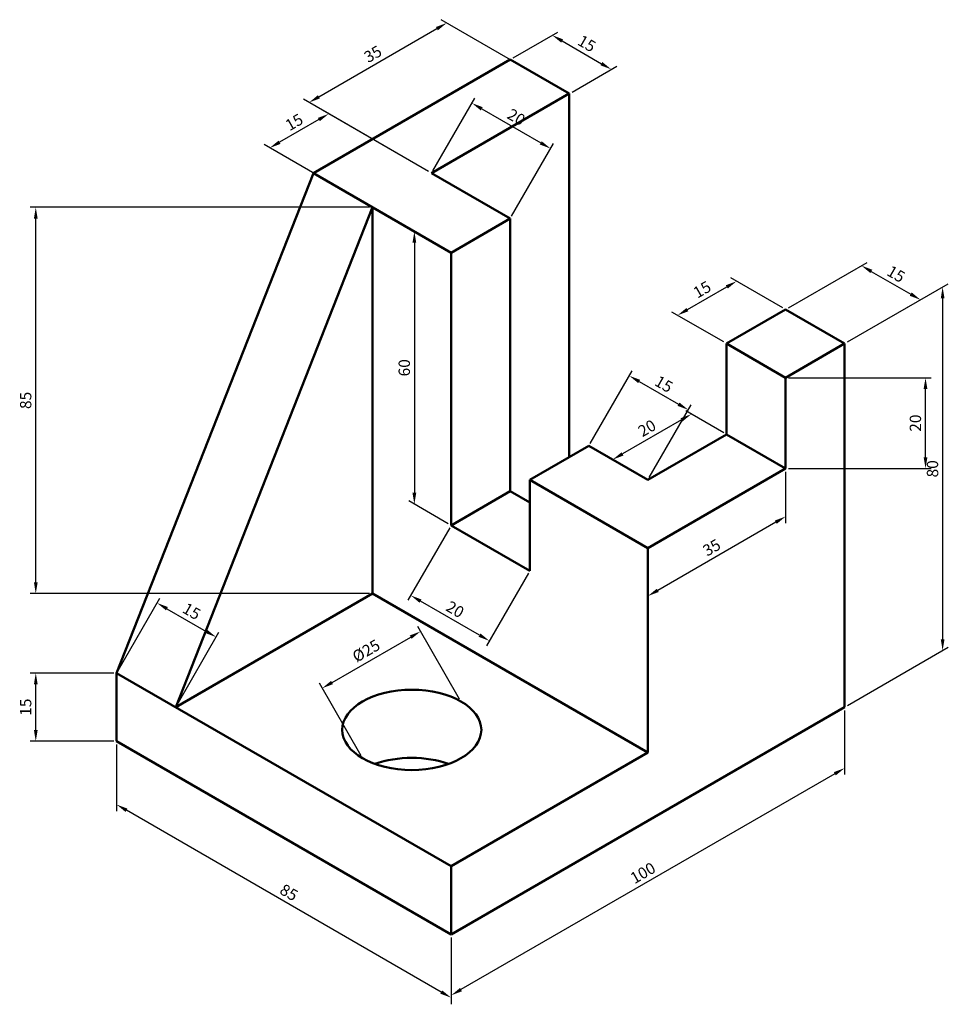
# Model space of a CAD drawing. Units: millimetres. Extents: x 1462 to 1666, y 2377 to 2594.
import ezdxf

# ---------------------------------------------------------------- set-up
doc = ezdxf.new("R2010")
doc.units = ezdxf.units.MM
doc.layers.add('M-DIMS', color=2, linetype='Continuous', lineweight=25)
doc.layers.add('M-OUTL', color=7, linetype='Continuous', lineweight=50)
doc.styles.get("Standard").update_dxf_attribs({"font": 'arial.ttf'})
doc.dimstyles.new('ISO-25', dxfattribs={"dimtxt": 2.5, "dimasz": 2.5, "dimexe": 1.25, "dimexo": 0.625, "dimtad": 1, "dimtxsty": 'Standard', "dimcen": 2.5, "dimadec": 0, "dimazin": 0, "dimtfac": 1, "dimtmove": 0, "dimatfit": 3, "dimfxl": 1, "dimarcsym": 0})

# ---------------------------------------------------------------- blocks, each defined once
blk = doc.blocks.new('*D1')
at = {"layer": 'Defpoints', "color": 0, "transparency": 16777216}
for p in [(1643.58, 2522.67), (1665.14, 2455.12), (1643.58, 2442.67)]:
    blk.add_point(p, dxfattribs=at)
at = {"layer": 'M-DIMS', "color": 0, "lineweight": -2, "transparency": 16777216}
for p, q in [((1644.2, 2523.03), (1666.39, 2535.85)), ((1665.14, 2532.62), (1665.14, 2457.62)), ((1644.2, 2443.03), (1666.39, 2455.85))]:
    blk.add_line(p, q, dxfattribs=at)
at = {"layer": 'M-DIMS', "color": 0, "transparency": 16777216}
for points in [[(1664.73, 2532.62), (1665.56, 2532.62), (1665.14, 2535.12)], [(1664.73, 2457.62), (1665.56, 2457.62), (1665.14, 2455.12)]]:
    blk.add_solid(points, dxfattribs=at)
at = {"layer": 'M-DIMS', "color": 0, "transparency": 16777216, "insert": (1663.24, 2495.12), "char_height": 2.5, "attachment_point": 5, "rotation": 90}
blk.add_mtext('80', dxfattribs=at)
blk = doc.blocks.new('*D2')
at = {"layer": 'Defpoints', "color": 0, "transparency": 16777216}
for p in [(1660.28, 2532.31), (1630.59, 2530.17), (1643.58, 2522.67)]:
    blk.add_point(p, dxfattribs=at)
at = {"layer": 'M-DIMS', "color": 0, "lineweight": -2, "transparency": 16777216}
for p, q in [((1631.21, 2530.53), (1648.54, 2540.54)), ((1649.45, 2538.56), (1658.11, 2533.56)), ((1644.2, 2523.03), (1661.53, 2533.04))]:
    blk.add_line(p, q, dxfattribs=at)
at = {"layer": 'M-DIMS', "color": 0, "transparency": 16777216}
for points in [[(1649.66, 2538.93), (1649.24, 2538.2), (1647.29, 2539.81)], [(1658.32, 2533.93), (1657.9, 2533.2), (1660.28, 2532.31)]]:
    blk.add_solid(points, dxfattribs=at)
at = {"layer": 'M-DIMS', "color": 0, "transparency": 16777216, "insert": (1654.73, 2537.71), "char_height": 2.5, "attachment_point": 5, "rotation": 330}
blk.add_mtext('15', dxfattribs=at)
blk = doc.blocks.new('*D3')
at = {"layer": 'Defpoints', "color": 0, "transparency": 16777216}
for p in [(1619.8, 2536.4), (1630.59, 2530.17), (1617.6, 2522.67)]:
    blk.add_point(p, dxfattribs=at)
at = {"layer": 'M-DIMS', "color": 0, "lineweight": -2, "transparency": 16777216}
for p, q in [((1608.98, 2530.15), (1617.64, 2535.15)), ((1629.96, 2530.53), (1618.55, 2537.12)), ((1616.97, 2523.03), (1605.56, 2529.62))]:
    blk.add_line(p, q, dxfattribs=at)
at = {"layer": 'M-DIMS', "color": 0, "transparency": 16777216}
for points in [[(1617.43, 2535.51), (1617.85, 2534.79), (1619.8, 2536.4)], [(1608.77, 2530.51), (1609.19, 2529.79), (1606.81, 2528.9)]]:
    blk.add_solid(points, dxfattribs=at)
at = {"layer": 'M-DIMS', "color": 0, "transparency": 16777216, "insert": (1612.36, 2534.3), "char_height": 2.5, "attachment_point": 5, "rotation": 30}
blk.add_mtext('15', dxfattribs=at)
blk = doc.blocks.new('*D4')
at = {"layer": 'Defpoints', "color": 0, "transparency": 16777216}
for p in [(1617.6, 2502.67), (1592.53, 2497.15), (1600.28, 2492.67)]:
    blk.add_point(p, dxfattribs=at)
at = {"layer": 'M-DIMS', "color": 0, "lineweight": -2, "transparency": 16777216}
for p, q in [((1616.97, 2503.03), (1608.6, 2507.87)), ((1607.68, 2505.9), (1594.69, 2498.4)), ((1599.65, 2493.03), (1591.28, 2497.87))]:
    blk.add_line(p, q, dxfattribs=at)
at = {"layer": 'M-DIMS', "color": 0, "transparency": 16777216}
for points in [[(1607.48, 2506.26), (1607.89, 2505.54), (1609.85, 2507.15)], [(1594.49, 2498.76), (1594.9, 2498.04), (1592.53, 2497.15)]]:
    blk.add_solid(points, dxfattribs=at)
at = {"layer": 'M-DIMS', "color": 0, "transparency": 16777216, "insert": (1600.24, 2503.79), "char_height": 2.5, "attachment_point": 5, "rotation": 30}
blk.add_mtext('20', dxfattribs=at)
blk = doc.blocks.new('*D5')
at = {"layer": 'Defpoints', "color": 0, "transparency": 16777216}
for p in [(1517.05, 2565.73), (1552.65, 2560.17), (1539.66, 2552.67)]:
    blk.add_point(p, dxfattribs=at)
at = {"layer": 'M-DIMS', "color": 0, "lineweight": -2, "transparency": 16777216}
for p, q in [((1527.87, 2571.98), (1519.21, 2566.98)), ((1552.02, 2560.53), (1528.79, 2573.95)), ((1539.03, 2553.03), (1515.8, 2566.45))]:
    blk.add_line(p, q, dxfattribs=at)
at = {"layer": 'M-DIMS', "color": 0, "transparency": 16777216}
for points in [[(1527.66, 2572.34), (1528.08, 2571.62), (1530.04, 2573.23)], [(1519, 2567.34), (1519.42, 2566.62), (1517.05, 2565.73)]]:
    blk.add_solid(points, dxfattribs=at)
at = {"layer": 'M-DIMS', "color": 0, "transparency": 16777216, "insert": (1522.59, 2571.12), "char_height": 2.5, "attachment_point": 5, "rotation": 30}
blk.add_mtext('15', dxfattribs=at)
blk = doc.blocks.new('*D6')
at = {"layer": 'Defpoints', "color": 0, "transparency": 16777216}
for p in [(1556.02, 2593.23), (1582.96, 2577.67), (1552.65, 2560.17)]:
    blk.add_point(p, dxfattribs=at)
at = {"layer": 'M-DIMS', "color": 0, "lineweight": -2, "transparency": 16777216}
for p, q in [((1582.33, 2578.03), (1554.77, 2593.95)), ((1527.87, 2576.98), (1553.85, 2591.98)), ((1552.02, 2560.53), (1524.46, 2576.45))]:
    blk.add_line(p, q, dxfattribs=at)
at = {"layer": 'M-DIMS', "color": 0, "transparency": 16777216}
for points in [[(1553.64, 2592.34), (1554.06, 2591.62), (1556.02, 2593.23)], [(1527.66, 2577.34), (1528.08, 2576.62), (1525.71, 2575.73)]]:
    blk.add_solid(points, dxfattribs=at)
at = {"layer": 'M-DIMS', "color": 0, "transparency": 16777216, "insert": (1539.91, 2586.12), "char_height": 2.5, "attachment_point": 5, "rotation": 30}
blk.add_mtext('35', dxfattribs=at)
blk = doc.blocks.new('*D7')
at = {"layer": 'Defpoints', "color": 0, "transparency": 16777216}
for p in [(1569.97, 2585.17), (1592.22, 2583.02), (1582.96, 2577.67)]:
    blk.add_point(p, dxfattribs=at)
at = {"layer": 'M-DIMS', "color": 0, "lineweight": -2, "transparency": 16777216}
for p, q in [((1570.59, 2585.53), (1580.48, 2591.24)), ((1581.39, 2589.27), (1590.05, 2584.27)), ((1583.58, 2578.03), (1593.47, 2583.74))]:
    blk.add_line(p, q, dxfattribs=at)
at = {"layer": 'M-DIMS', "color": 0, "transparency": 16777216}
for points in [[(1581.6, 2589.63), (1581.19, 2588.91), (1579.23, 2590.52)], [(1590.26, 2584.63), (1589.85, 2583.91), (1592.22, 2583.02)]]:
    blk.add_solid(points, dxfattribs=at)
at = {"layer": 'M-DIMS', "color": 0, "transparency": 16777216, "insert": (1586.68, 2588.42), "char_height": 2.5, "attachment_point": 5, "rotation": 330}
blk.add_mtext('15', dxfattribs=at)
blk = doc.blocks.new('*D8')
at = {"layer": 'Defpoints', "color": 0, "transparency": 16777216}
for p in [(1556.98, 2542.67), (1548.88, 2487.35), (1556.98, 2482.67)]:
    blk.add_point(p, dxfattribs=at)
at = {"layer": 'M-DIMS', "color": 0, "lineweight": -2, "transparency": 16777216}
for p, q in [((1556.35, 2543.03), (1547.63, 2548.07)), ((1548.88, 2544.85), (1548.88, 2489.85)), ((1556.35, 2483.03), (1547.63, 2488.07))]:
    blk.add_line(p, q, dxfattribs=at)
at = {"layer": 'M-DIMS', "color": 0, "transparency": 16777216}
for points in [[(1548.46, 2544.85), (1549.3, 2544.85), (1548.88, 2547.35)], [(1548.46, 2489.85), (1549.3, 2489.85), (1548.88, 2487.35)]]:
    blk.add_solid(points, dxfattribs=at)
at = {"layer": 'M-DIMS', "color": 0, "transparency": 16777216, "insert": (1546.98, 2517.35), "char_height": 2.5, "attachment_point": 5, "rotation": 90}
blk.add_mtext('60', dxfattribs=at)
blk = doc.blocks.new('*D9')
at = {"layer": 'Defpoints', "color": 0, "transparency": 16777216}
for p in [(1630.59, 2495.17), (1600.28, 2477.67), (1600.28, 2467.12)]:
    blk.add_point(p, dxfattribs=at)
at = {"layer": 'M-DIMS', "color": 0, "lineweight": -2, "transparency": 16777216}
for p, q in [((1630.59, 2494.45), (1630.59, 2483.17)), ((1628.42, 2483.37), (1602.44, 2468.37)), ((1600.28, 2476.95), (1600.28, 2465.67))]:
    blk.add_line(p, q, dxfattribs=at)
at = {"layer": 'M-DIMS', "color": 0, "transparency": 16777216}
for points in [[(1628.21, 2483.73), (1628.63, 2483.01), (1630.59, 2484.62)], [(1602.23, 2468.73), (1602.65, 2468.01), (1600.28, 2467.12)]]:
    blk.add_solid(points, dxfattribs=at)
at = {"layer": 'M-DIMS', "color": 0, "transparency": 16777216, "insert": (1614.48, 2477.52), "char_height": 2.5, "attachment_point": 5, "rotation": 30}
blk.add_mtext('35', dxfattribs=at)
blk = doc.blocks.new('*D10')
at = {"layer": 'Defpoints', "color": 0, "transparency": 16777216}
for p in [(1643.58, 2442.67), (1556.98, 2392.67), (1556.98, 2379.26)]:
    blk.add_point(p, dxfattribs=at)
at = {"layer": 'M-DIMS', "color": 0, "lineweight": -2, "transparency": 16777216}
for p, q in [((1643.58, 2441.95), (1643.58, 2427.82)), ((1641.41, 2428.01), (1559.14, 2380.51)), ((1556.98, 2391.95), (1556.98, 2377.82))]:
    blk.add_line(p, q, dxfattribs=at)
at = {"layer": 'M-DIMS', "color": 0, "transparency": 16777216}
for points in [[(1641.2, 2428.37), (1641.62, 2427.65), (1643.58, 2429.26)], [(1558.93, 2380.87), (1559.35, 2380.15), (1556.98, 2379.26)]]:
    blk.add_solid(points, dxfattribs=at)
at = {"layer": 'M-DIMS', "color": 0, "transparency": 16777216, "insert": (1599.33, 2405.91), "char_height": 2.5, "attachment_point": 5, "rotation": 30}
blk.add_mtext('100', dxfattribs=at)
blk = doc.blocks.new('*D11')
at = {"layer": 'Defpoints', "color": 0, "transparency": 16777216}
for p in [(1483.36, 2435.17), (1483.36, 2421.23), (1556.98, 2392.67)]:
    blk.add_point(p, dxfattribs=at)
at = {"layer": 'M-DIMS', "color": 0, "lineweight": -2, "transparency": 16777216}
for p, q in [((1483.36, 2434.45), (1483.36, 2419.78)), ((1554.81, 2379.98), (1485.53, 2419.98)), ((1556.98, 2391.95), (1556.98, 2377.28))]:
    blk.add_line(p, q, dxfattribs=at)
at = {"layer": 'M-DIMS', "color": 0, "transparency": 16777216}
for points in [[(1485.74, 2420.34), (1485.32, 2419.62), (1483.36, 2421.23)], [(1555.02, 2380.34), (1554.6, 2379.62), (1556.98, 2378.73)]]:
    blk.add_solid(points, dxfattribs=at)
at = {"layer": 'M-DIMS', "color": 0, "transparency": 16777216, "insert": (1521.12, 2401.62), "char_height": 2.5, "attachment_point": 5, "rotation": 330}
blk.add_mtext('85', dxfattribs=at)
blk = doc.blocks.new('*D12')
at = {"layer": 'Defpoints', "color": 0, "transparency": 16777216}
for p in [(1550.24, 2459.34), (1559.14, 2443.92), (1537.49, 2431.42)]:
    blk.add_point(p, dxfattribs=at)
at = {"layer": 'M-DIMS', "color": 0, "lineweight": -2, "transparency": 16777216}
for p, q in [((1558.83, 2444.46), (1549.62, 2460.42)), ((1530.76, 2448.09), (1548.08, 2458.09)), ((1537.18, 2431.96), (1527.97, 2447.92))]:
    blk.add_line(p, q, dxfattribs=at)
at = {"layer": 'M-DIMS', "color": 0, "transparency": 16777216}
for points in [[(1547.87, 2458.45), (1548.28, 2457.73), (1550.24, 2459.34)], [(1530.55, 2448.45), (1530.96, 2447.73), (1528.59, 2446.84)]]:
    blk.add_solid(points, dxfattribs=at)
at = {"layer": 'M-DIMS', "color": 0, "transparency": 16777216, "insert": (1538.43, 2454.8), "char_height": 2.5, "attachment_point": 5, "rotation": 30}
blk.add_mtext('%%c25', dxfattribs=at)
blk = doc.blocks.new('*D13')
at = {"layer": 'Defpoints', "color": 0, "transparency": 16777216}
for p in [(1465.56, 2450.17), (1483.36, 2450.17), (1483.36, 2435.17)]:
    blk.add_point(p, dxfattribs=at)
at = {"layer": 'M-DIMS', "color": 0, "lineweight": -2, "transparency": 16777216}
for p, q in [((1482.74, 2450.17), (1464.31, 2450.17)), ((1465.56, 2437.67), (1465.56, 2447.67)), ((1482.74, 2435.17), (1464.31, 2435.17))]:
    blk.add_line(p, q, dxfattribs=at)
at = {"layer": 'M-DIMS', "color": 0, "transparency": 16777216}
for points in [[(1465.15, 2447.67), (1465.98, 2447.67), (1465.56, 2450.17)], [(1465.15, 2437.67), (1465.98, 2437.67), (1465.56, 2435.17)]]:
    blk.add_solid(points, dxfattribs=at)
at = {"layer": 'M-DIMS', "color": 0, "transparency": 16777216, "insert": (1463.66, 2442.67), "char_height": 2.5, "attachment_point": 5, "rotation": 90}
blk.add_mtext('15', dxfattribs=at)
blk = doc.blocks.new('*D14')
at = {"layer": 'Defpoints', "color": 0, "transparency": 16777216}
for p in [(1465.56, 2552.67), (1539.66, 2552.67), (1539.66, 2467.67)]:
    blk.add_point(p, dxfattribs=at)
at = {"layer": 'M-DIMS', "color": 0, "lineweight": -2, "transparency": 16777216}
for p, q in [((1539.03, 2552.67), (1464.31, 2552.67)), ((1465.56, 2470.17), (1465.56, 2550.17)), ((1539.03, 2467.67), (1464.31, 2467.67))]:
    blk.add_line(p, q, dxfattribs=at)
at = {"layer": 'M-DIMS', "color": 0, "transparency": 16777216}
for points in [[(1465.15, 2550.17), (1465.98, 2550.17), (1465.56, 2552.67)], [(1465.15, 2470.17), (1465.98, 2470.17), (1465.56, 2467.67)]]:
    blk.add_solid(points, dxfattribs=at)
at = {"layer": 'M-DIMS', "color": 0, "transparency": 16777216, "insert": (1463.66, 2510.17), "char_height": 2.5, "attachment_point": 5, "rotation": 90}
blk.add_mtext('85', dxfattribs=at)
blk = doc.blocks.new('*D15')
at = {"layer": 'Defpoints', "color": 0, "transparency": 16777216}
for p in [(1505.25, 2458.09), (1483.36, 2450.17), (1496.35, 2442.67)]:
    blk.add_point(p, dxfattribs=at)
at = {"layer": 'M-DIMS', "color": 0, "lineweight": -2, "transparency": 16777216}
for p, q in [((1483.68, 2450.71), (1492.89, 2466.67)), ((1494.43, 2464.34), (1503.09, 2459.34)), ((1496.67, 2443.21), (1505.88, 2459.17))]:
    blk.add_line(p, q, dxfattribs=at)
at = {"layer": 'M-DIMS', "color": 0, "transparency": 16777216}
for points in [[(1494.64, 2464.7), (1494.22, 2463.98), (1492.26, 2465.59)], [(1503.3, 2459.7), (1502.88, 2458.98), (1505.25, 2458.09)]]:
    blk.add_solid(points, dxfattribs=at)
at = {"layer": 'M-DIMS', "color": 0, "transparency": 16777216, "insert": (1499.71, 2463.49), "char_height": 2.5, "attachment_point": 5, "rotation": 330}
blk.add_mtext('15', dxfattribs=at)
blk = doc.blocks.new('*D16')
at = {"layer": 'Defpoints', "color": 0, "transparency": 16777216}
for p in [(1578.87, 2565.59), (1552.65, 2560.17), (1569.97, 2550.17)]:
    blk.add_point(p, dxfattribs=at)
at = {"layer": 'M-DIMS', "color": 0, "lineweight": -2, "transparency": 16777216}
for p, q in [((1552.96, 2560.71), (1562.17, 2576.67)), ((1563.71, 2574.34), (1576.7, 2566.84)), ((1570.28, 2550.71), (1579.49, 2566.67))]:
    blk.add_line(p, q, dxfattribs=at)
at = {"layer": 'M-DIMS', "color": 0, "transparency": 16777216}
for points in [[(1563.92, 2574.7), (1563.5, 2573.98), (1561.55, 2575.59)], [(1576.91, 2567.2), (1576.49, 2566.48), (1578.87, 2565.59)]]:
    blk.add_solid(points, dxfattribs=at)
at = {"layer": 'M-DIMS', "color": 0, "transparency": 16777216, "insert": (1571.16, 2572.24), "char_height": 2.5, "attachment_point": 5, "rotation": 330}
blk.add_mtext('20', dxfattribs=at)
blk = doc.blocks.new('*D17')
at = {"layer": 'Defpoints', "color": 0, "transparency": 16777216}
for p in [(1556.98, 2482.67), (1574.3, 2472.67), (1548.08, 2467.26)]:
    blk.add_point(p, dxfattribs=at)
at = {"layer": 'M-DIMS', "color": 0, "lineweight": -2, "transparency": 16777216}
for p, q in [((1556.66, 2482.13), (1547.45, 2466.18)), ((1573.98, 2472.13), (1564.77, 2456.18)), ((1563.23, 2458.51), (1550.24, 2466.01))]:
    blk.add_line(p, q, dxfattribs=at)
at = {"layer": 'M-DIMS', "color": 0, "transparency": 16777216}
for points in [[(1550.45, 2466.37), (1550.03, 2465.65), (1548.08, 2467.26)], [(1563.44, 2458.87), (1563.02, 2458.15), (1565.4, 2457.26)]]:
    blk.add_solid(points, dxfattribs=at)
at = {"layer": 'M-DIMS', "color": 0, "transparency": 16777216, "insert": (1557.69, 2463.91), "char_height": 2.5, "attachment_point": 5, "rotation": 330}
blk.add_mtext('20', dxfattribs=at)
blk = doc.blocks.new('*D18')
at = {"layer": 'Defpoints', "color": 0, "transparency": 16777216}
for p in [(1630.59, 2515.17), (1661.38, 2515.17), (1630.59, 2495.17)]:
    blk.add_point(p, dxfattribs=at)
at = {"layer": 'M-DIMS', "color": 0, "lineweight": -2, "transparency": 16777216}
for p, q in [((1631.21, 2515.17), (1662.63, 2515.17)), ((1661.38, 2497.67), (1661.38, 2512.67)), ((1631.21, 2495.17), (1662.63, 2495.17))]:
    blk.add_line(p, q, dxfattribs=at)
at = {"layer": 'M-DIMS', "color": 0, "transparency": 16777216}
for points in [[(1660.96, 2512.67), (1661.79, 2512.67), (1661.38, 2515.17)], [(1660.96, 2497.67), (1661.79, 2497.67), (1661.38, 2495.17)]]:
    blk.add_solid(points, dxfattribs=at)
at = {"layer": 'M-DIMS', "color": 0, "transparency": 16777216, "insert": (1659.48, 2505.17), "char_height": 2.5, "attachment_point": 5, "rotation": 90}
blk.add_mtext('20', dxfattribs=at)
blk = doc.blocks.new('*D19')
at = {"layer": 'Defpoints', "color": 0, "transparency": 16777216}
for p in [(1609.18, 2508.09), (1587.29, 2500.17), (1600.28, 2492.67)]:
    blk.add_point(p, dxfattribs=at)
at = {"layer": 'M-DIMS', "color": 0, "lineweight": -2, "transparency": 16777216}
for p, q in [((1587.6, 2500.71), (1596.81, 2516.67)), ((1598.35, 2514.34), (1607.01, 2509.34)), ((1600.59, 2493.21), (1609.8, 2509.17))]:
    blk.add_line(p, q, dxfattribs=at)
at = {"layer": 'M-DIMS', "color": 0, "transparency": 16777216}
for points in [[(1598.56, 2514.7), (1598.14, 2513.98), (1596.19, 2515.59)], [(1607.22, 2509.7), (1606.8, 2508.98), (1609.18, 2508.09)]]:
    blk.add_solid(points, dxfattribs=at)
at = {"layer": 'M-DIMS', "color": 0, "transparency": 16777216, "insert": (1603.63, 2513.49), "char_height": 2.5, "attachment_point": 5, "rotation": 330}
blk.add_mtext('15', dxfattribs=at)

msp = doc.modelspace()

# ---------------------------------------------------------------- linework, layer by layer
at = {"layer": 'M-OUTL'}
for p, q in [((1526.665, 2560.174), (1569.966, 2585.174)), ((1569.966, 2585.174), (1582.956, 2577.674)), ((1582.956, 2577.674), (1552.646, 2560.174)), ((1582.956, 2577.674), (1582.956, 2497.674)), ((1526.665, 2560.174), (1483.364, 2450.174)), ((1556.976, 2542.674), (1526.665, 2560.174)), ((1552.646, 2560.174), (1569.966, 2550.174)), ((1496.354, 2442.674), (1539.655, 2552.674)), ((1539.655, 2552.674), (1539.655, 2467.674)), ((1556.976, 2542.674), (1569.966, 2550.174)), ((1569.966, 2550.174), (1569.966, 2490.174)), ((1556.976, 2482.674), (1556.976, 2542.674)), ((1630.588, 2530.174), (1617.597, 2522.674)), ((1643.578, 2522.674), (1630.588, 2530.174)), ((1617.597, 2522.674), (1617.597, 2502.674)), ((1630.588, 2515.174), (1617.597, 2522.674)), ((1630.588, 2515.174), (1643.578, 2522.674)), ((1643.578, 2522.674), (1643.578, 2442.674)), ((1630.588, 2495.174), (1630.588, 2515.174)), ((1617.597, 2502.674), (1600.277, 2492.674)), ((1617.597, 2502.674), (1630.588, 2495.174)), ((1587.287, 2500.174), (1574.296, 2492.674)), ((1600.277, 2492.674), (1587.287, 2500.174)), ((1600.277, 2477.674), (1630.588, 2495.174)), ((1600.277, 2477.674), (1574.296, 2492.674)), ((1574.296, 2492.674), (1574.296, 2472.674)), ((1569.966, 2490.174), (1556.976, 2482.674)), ((1569.966, 2490.174), (1574.296, 2487.674)), ((1574.296, 2472.674), (1556.976, 2482.674)), ((1600.277, 2432.674), (1600.277, 2477.674)), ((1496.354, 2442.674), (1539.655, 2467.674)), ((1539.655, 2467.674), (1600.277, 2432.674)), ((1483.364, 2435.174), (1483.364, 2450.174)), ((1483.364, 2450.174), (1556.976, 2407.674)), ((1643.578, 2442.674), (1556.976, 2392.674)), ((1556.976, 2392.674), (1483.364, 2435.174)), ((1556.976, 2407.674), (1600.277, 2432.674)), ((1556.976, 2407.674), (1556.976, 2392.674))]:
    msp.add_line(p, q, dxfattribs=at)
msp.add_ellipse((1548.315, 2437.674), major_axis=(-15.309, 0), ratio=0.5773503, dxfattribs=at)
msp.add_ellipse((1548.315, 2422.674), major_axis=(-15.309, 0), ratio=0.5773503, start_param=4.1547902, end_param=5.2699878, dxfattribs=at)

# ---------------------------------------------------------------- dimensions: what is measured, and where the dimension line sits
at = {"layer": 'M-DIMS'}
for p1, p2, distance, picture, middle in [((1552.646, 2560.174), (1582.956, 2577.674), 26.94, '*D6', (1539.91, 2586.125)), ((1569.966, 2585.174), (1582.956, 2577.674), 9.263, '*D7', (1586.675, 2588.418)), ((1552.646, 2560.174), (1539.655, 2552.674), -22.609, '*D5', (1522.591, 2571.124)), ((1556.976, 2542.674), (1556.976, 2482.674), -8.096, '*D8', (1546.978, 2517.348)), ((1630.588, 2530.174), (1643.578, 2522.674), 16.698, '*D2', (1654.732, 2537.711)), ((1617.597, 2522.674), (1630.588, 2530.174), 10.785, '*D3', (1612.357, 2534.297)), ((1643.578, 2522.674), (1643.578, 2442.674), 21.565, '*D1', (1663.242, 2495.124)), ((1617.597, 2502.674), (1600.277, 2492.674), -7.748, '*D4', (1600.238, 2503.794)), ((1630.588, 2495.174), (1600.277, 2477.674), 9.142, '*D9', (1614.481, 2477.515)), ((1643.578, 2442.674), (1556.976, 2392.674), 11.618, '*D10', (1599.326, 2405.906)), ((1556.976, 2392.674), (1483.364, 2435.174), 12.078, '*D11', (1521.12, 2401.623))]:
    dim = msp.add_aligned_dim(p1=p1, p2=p2, distance=distance, dimstyle='ISO-25', override={"dimclrd": 0, "dimclre": 0, "dimclrt": 0}, dxfattribs=at)
    dim.commit()
    dim.dimension.update_dxf_attribs({"geometry": picture, "text_midpoint": middle})
for base, p1, p2, angle, picture, middle in [((1578.866, 2565.589), (1552.646, 2560.174), (1569.966, 2550.174), 330, '*D16', (1571.157, 2572.236)), ((1465.564, 2552.674), (1539.655, 2467.674), (1539.655, 2552.674), 90, '*D14', (1463.662, 2510.174)), ((1609.177, 2508.089), (1587.287, 2500.174), (1600.277, 2492.674), 330, '*D19', (1603.632, 2513.486)), ((1661.378, 2515.174), (1630.588, 2495.174), (1630.588, 2515.174), 90, '*D18', (1659.477, 2505.174)), ((1548.076, 2467.258), (1574.296, 2472.674), (1556.976, 2482.674), 150, '*D17', (1557.687, 2463.905)), ((1505.254, 2458.089), (1483.364, 2450.174), (1496.354, 2442.674), 330, '*D15', (1499.709, 2463.486)), ((1465.564, 2450.174), (1483.364, 2435.174), (1483.364, 2450.174), 90, '*D13', (1463.662, 2442.674))]:
    dim = msp.add_linear_dim(base=base, p1=p1, p2=p2, angle=angle, dimstyle='ISO-25', override={"dimdec": 0, "dimlfac": 1, "dimrnd": 0, "dimzin": 0, "dimdsep": 46, "dimlunit": 2}, dxfattribs=at)
    dim.commit()
    dim.dimension.update_dxf_attribs({"geometry": picture, "text_midpoint": middle})
dim = msp.add_linear_dim(base=(1550.241, 2459.339), p1=(1537.49, 2431.424), p2=(1559.141, 2443.924), angle=30, text='%%c<>', dimstyle='ISO-25', override={"dimdec": 0, "dimlfac": 1, "dimrnd": 0, "dimzin": 0, "dimdsep": 46, "dimlunit": 2}, dxfattribs=at)
dim.commit()
dim.dimension.update_dxf_attribs({"geometry": '*D12', "text_midpoint": (1538.43, 2454.796)})

doc.saveas('drawing.dxf')
